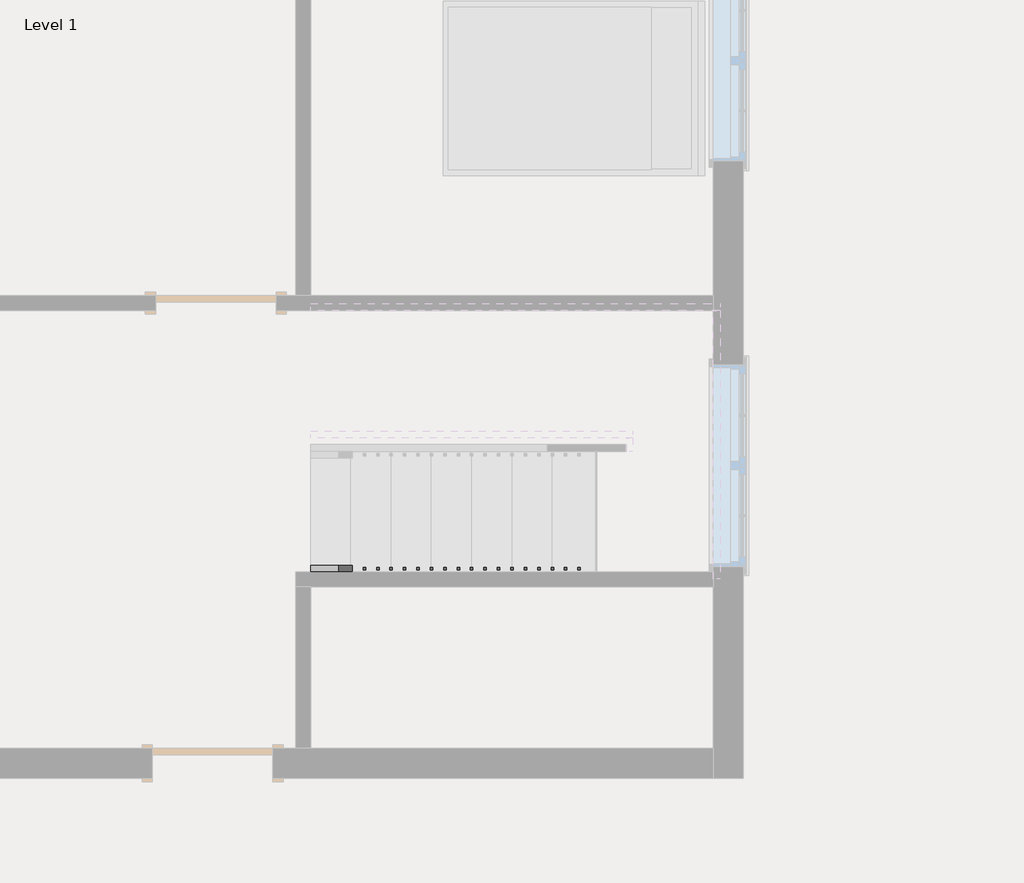
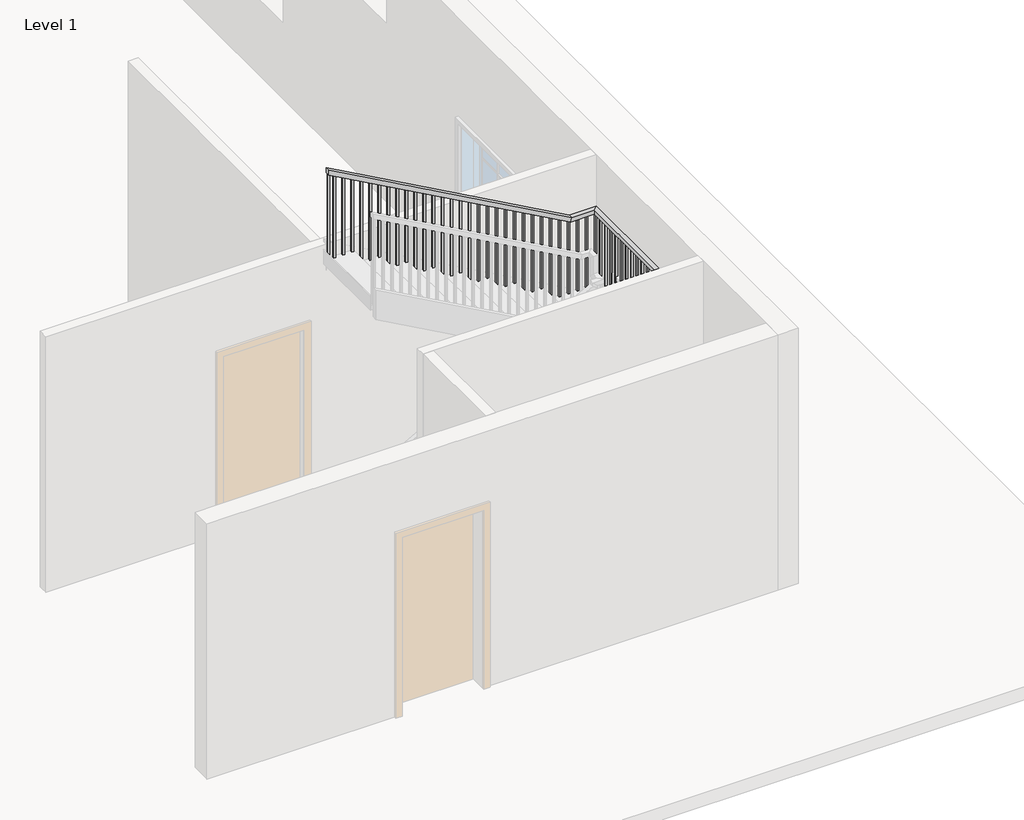
# One storey, part 2 of 3: 1 railing.
"""IFC4 building model written with IfcOpenShell, lengths in millimetres."""

from ifc_helpers import new_model, si_unit, frame, origin, place, context, project, spatial, polyline, outline, extrude, faceted_brep, element, save

model = new_model("IFC4")

# Units and contexts
model_context = context("Model", 3, world=origin())
ifc_project = project(units=[si_unit("LENGTHUNIT", "METRE", prefix="MILLI")], contexts=[model_context])

# Site, building, storey
site = spatial("IfcSite", under=ifc_project)
building = spatial("IfcBuilding", under=site)
storey = spatial("IfcBuildingStorey", under=building, Name="Level 1", Elevation=0.0)

# Railing
placement = place(None, origin())
element("IfcRailing", 1, ObjectType="Handrail - Rectangular", at=placement, inside=storey, context=model_context, shape_type="SolidModel", body=[
    faceted_brep([(-1197.97188, -4765.70869, 1083.7333333), (-1197.97188, -4765.70869, 1025.620221), (-1197.97188, -4816.50869, 1025.620221), (-1197.97188, -4816.50869, 1083.7333333), (1240.42812, -4765.70869, 2438.4), (1253.5917222, -4765.70869, 2387.6), (1253.5917222, -4816.50869, 2387.6), (1240.42812, -4816.50869, 2438.4), (1799.22812, -4765.70869, 2438.4), (1799.22812, -4765.70869, 2387.6), (1850.02812, -4816.50869, 2387.6), (1850.02812, -4816.50869, 2438.4), (1799.22812, -2886.10869, 2438.4), (1799.22812, -2886.10869, 2387.6), (1850.02812, -2835.30869, 2387.6), (1850.02812, -2835.30869, 2438.4), (1545.22812, -2886.10869, 2438.4), (1532.0645177, -2886.10869, 2387.6), (1532.0645177, -2835.30869, 2387.6), (1545.22812, -2835.30869, 2438.4), (-1197.97188, -2886.10869, 3962.4), (-1197.97188, -2835.30869, 3962.4), (-1197.97188, -2835.30869, 3904.2868876), (-1197.97188, -2886.10869, 3904.2868876)], [[[0, 1, 2, 3]], [[1, 0, 4, 5]], [[2, 1, 5, 6]], [[3, 2, 6, 7]], [[0, 3, 7, 4]], [[5, 4, 8, 9]], [[6, 5, 9, 10]], [[7, 6, 10, 11]], [[4, 7, 11, 8]], [[9, 8, 12, 13]], [[10, 9, 13, 14]], [[11, 10, 14, 15]], [[8, 11, 15, 12]], [[13, 12, 16, 17]], [[14, 13, 17, 18]], [[15, 14, 18, 19]], [[12, 15, 19, 16]], [[20, 21, 22, 23]], [[17, 16, 20, 23]], [[18, 17, 23, 22]], [[19, 18, 22, 21]], [[16, 19, 21, 20]]]),
    extrude(outline(polyline([(3856.6618876, -1112.24688), (3867.245221, -1131.29688), (2878.6666667, -1131.29688), (2878.6666667, -1112.24688), (3856.6618876, -1112.24688)])), frame((0.0, -2870.23369, 0.0), z_axis=(0.0, 1.0, 0.0), x_axis=(0.0, 0.0, 1.0)), (0.0, 0.0, 1.0), 19.05),
    extrude(outline(polyline([(3800.2174432, -1010.64688), (3810.8007765, -1029.69688), (2878.6666667, -1029.69688), (2878.6666667, -1010.64688), (3800.2174432, -1010.64688)])), frame((0.0, -2870.23369, 0.0), z_axis=(0.0, 1.0, 0.0), x_axis=(0.0, 0.0, 1.0)), (0.0, 0.0, 1.0), 19.05),
    extrude(outline(polyline([(3743.7729988, -909.04688), (3754.3563321, -928.09688), (2878.6666667, -928.09688), (2878.6666667, -909.04688), (3743.7729988, -909.04688)])), frame((0.0, -2870.23369, 0.0), z_axis=(0.0, 1.0, 0.0), x_axis=(0.0, 0.0, 1.0)), (0.0, 0.0, 1.0), 19.05),
    extrude(outline(polyline([(3687.3285543, -807.44688), (3697.9118876, -826.49688), (2709.3333333, -826.49688), (2709.3333333, -807.44688), (3687.3285543, -807.44688)])), frame((0.0, -2870.23369, 0.0), z_axis=(0.0, 1.0, 0.0), x_axis=(0.0, 0.0, 1.0)), (0.0, 0.0, 1.0), 19.05),
    extrude(outline(polyline([(3630.8841099, -705.84688), (3641.4674432, -724.89688), (2709.3333333, -724.89688), (2709.3333333, -705.84688), (3630.8841099, -705.84688)])), frame((0.0, -2870.23369, 0.0), z_axis=(0.0, 1.0, 0.0), x_axis=(0.0, 0.0, 1.0)), (0.0, 0.0, 1.0), 19.05),
    extrude(outline(polyline([(3574.4396654, -604.24688), (3585.0229988, -623.29688), (2709.3333333, -623.29688), (2709.3333333, -604.24688), (3574.4396654, -604.24688)])), frame((0.0, -2870.23369, 0.0), z_axis=(0.0, 1.0, 0.0), x_axis=(0.0, 0.0, 1.0)), (0.0, 0.0, 1.0), 19.05),
    extrude(outline(polyline([(3517.995221, -502.64688), (3528.5785543, -521.69688), (2540.0, -521.69688), (2540.0, -502.64688), (3517.995221, -502.64688)])), frame((0.0, -2870.23369, 0.0), z_axis=(0.0, 1.0, 0.0), x_axis=(0.0, 0.0, 1.0)), (0.0, 0.0, 1.0), 19.05),
    extrude(outline(polyline([(3461.5507765, -401.04688), (3472.1341099, -420.09688), (2540.0, -420.09688), (2540.0, -401.04688), (3461.5507765, -401.04688)])), frame((0.0, -2870.23369, 0.0), z_axis=(0.0, 1.0, 0.0), x_axis=(0.0, 0.0, 1.0)), (0.0, 0.0, 1.0), 19.05),
    extrude(outline(polyline([(3405.1063321, -299.44688), (3415.6896654, -318.49688), (2540.0, -318.49688), (2540.0, -299.44688), (3405.1063321, -299.44688)])), frame((0.0, -2870.23369, 0.0), z_axis=(0.0, 1.0, 0.0), x_axis=(0.0, 0.0, 1.0)), (0.0, 0.0, 1.0), 19.05),
    extrude(outline(polyline([(3348.6618876, -197.84688), (3359.245221, -216.89688), (2370.6666667, -216.89688), (2370.6666667, -197.84688), (3348.6618876, -197.84688)])), frame((0.0, -2870.23369, 0.0), z_axis=(0.0, 1.0, 0.0), x_axis=(0.0, 0.0, 1.0)), (0.0, 0.0, 1.0), 19.05),
    extrude(outline(polyline([(3292.2174432, -96.24688), (3302.8007765, -115.29688), (2370.6666667, -115.29688), (2370.6666667, -96.24688), (3292.2174432, -96.24688)])), frame((0.0, -2870.23369, 0.0), z_axis=(0.0, 1.0, 0.0), x_axis=(0.0, 0.0, 1.0)), (0.0, 0.0, 1.0), 19.05),
    extrude(outline(polyline([(3235.7729988, 5.35312), (3246.3563321, -13.69688), (2370.6666667, -13.69688), (2370.6666667, 5.35312), (3235.7729988, 5.35312)])), frame((0.0, -2870.23369, 0.0), z_axis=(0.0, 1.0, 0.0), x_axis=(0.0, 0.0, 1.0)), (0.0, 0.0, 1.0), 19.05),
    extrude(outline(polyline([(3179.3285543, 106.95312), (3189.9118876, 87.90312), (2201.3333333, 87.90312), (2201.3333333, 106.95312), (3179.3285543, 106.95312)])), frame((0.0, -2870.23369, 0.0), z_axis=(0.0, 1.0, 0.0), x_axis=(0.0, 0.0, 1.0)), (0.0, 0.0, 1.0), 19.05),
    extrude(outline(polyline([(3122.8841099, 208.55312), (3133.4674432, 189.50312), (2201.3333333, 189.50312), (2201.3333333, 208.55312), (3122.8841099, 208.55312)])), frame((0.0, -2870.23369, 0.0), z_axis=(0.0, 1.0, 0.0), x_axis=(0.0, 0.0, 1.0)), (0.0, 0.0, 1.0), 19.05),
    extrude(outline(polyline([(3066.4396654, 310.15312), (3077.0229988, 291.10312), (2201.3333333, 291.10312), (2201.3333333, 310.15312), (3066.4396654, 310.15312)])), frame((0.0, -2870.23369, 0.0), z_axis=(0.0, 1.0, 0.0), x_axis=(0.0, 0.0, 1.0)), (0.0, 0.0, 1.0), 19.05),
    extrude(outline(polyline([(3009.995221, 411.75312), (3020.5785543, 392.70312), (2032.0, 392.70312), (2032.0, 411.75312), (3009.995221, 411.75312)])), frame((0.0, -2870.23369, 0.0), z_axis=(0.0, 1.0, 0.0), x_axis=(0.0, 0.0, 1.0)), (0.0, 0.0, 1.0), 19.05),
    extrude(outline(polyline([(2953.5507765, 513.35312), (2964.1341099, 494.30312), (2032.0, 494.30312), (2032.0, 513.35312), (2953.5507765, 513.35312)])), frame((0.0, -2870.23369, 0.0), z_axis=(0.0, 1.0, 0.0), x_axis=(0.0, 0.0, 1.0)), (0.0, 0.0, 1.0), 19.05),
    extrude(outline(polyline([(2897.1063321, 614.95312), (2907.6896654, 595.90312), (2032.0, 595.90312), (2032.0, 614.95312), (2897.1063321, 614.95312)])), frame((0.0, -2870.23369, 0.0), z_axis=(0.0, 1.0, 0.0), x_axis=(0.0, 0.0, 1.0)), (0.0, 0.0, 1.0), 19.05),
    extrude(outline(polyline([(2840.6618876, 716.55312), (2851.245221, 697.50312), (1862.6666667, 697.50312), (1862.6666667, 716.55312), (2840.6618876, 716.55312)])), frame((0.0, -2870.23369, 0.0), z_axis=(0.0, 1.0, 0.0), x_axis=(0.0, 0.0, 1.0)), (0.0, 0.0, 1.0), 19.05),
    extrude(outline(polyline([(2784.2174432, 818.15312), (2794.8007765, 799.10312), (1862.6666667, 799.10312), (1862.6666667, 818.15312), (2784.2174432, 818.15312)])), frame((0.0, -2870.23369, 0.0), z_axis=(0.0, 1.0, 0.0), x_axis=(0.0, 0.0, 1.0)), (0.0, 0.0, 1.0), 19.05),
    extrude(outline(polyline([(2727.7729988, 919.75312), (2738.3563321, 900.70312), (1862.6666667, 900.70312), (1862.6666667, 919.75312), (2727.7729988, 919.75312)])), frame((0.0, -2870.23369, 0.0), z_axis=(0.0, 1.0, 0.0), x_axis=(0.0, 0.0, 1.0)), (0.0, 0.0, 1.0), 19.05),
    extrude(outline(polyline([(2671.3285543, 1021.35312), (2681.9118876, 1002.30312), (1693.3333333, 1002.30312), (1693.3333333, 1021.35312), (2671.3285543, 1021.35312)])), frame((0.0, -2870.23369, 0.0), z_axis=(0.0, 1.0, 0.0), x_axis=(0.0, 0.0, 1.0)), (0.0, 0.0, 1.0), 19.05),
    extrude(outline(polyline([(2614.8841099, 1122.95312), (2625.4674432, 1103.90312), (1693.3333333, 1103.90312), (1693.3333333, 1122.95312), (2614.8841099, 1122.95312)])), frame((0.0, -2870.23369, 0.0), z_axis=(0.0, 1.0, 0.0), x_axis=(0.0, 0.0, 1.0)), (0.0, 0.0, 1.0), 19.05),
    extrude(outline(polyline([(2558.4396654, 1224.55312), (2569.0229988, 1205.50312), (1693.3333333, 1205.50312), (1693.3333333, 1224.55312), (2558.4396654, 1224.55312)])), frame((0.0, -2870.23369, 0.0), z_axis=(0.0, 1.0, 0.0), x_axis=(0.0, 0.0, 1.0)), (0.0, 0.0, 1.0), 19.05),
    extrude(outline(polyline([(2501.995221, 1326.15312), (2512.5785543, 1307.10312), (1524.0, 1307.10312), (1524.0, 1326.15312), (2501.995221, 1326.15312)])), frame((0.0, -2870.23369, 0.0), z_axis=(0.0, 1.0, 0.0), x_axis=(0.0, 0.0, 1.0)), (0.0, 0.0, 1.0), 19.05),
    extrude(outline(polyline([(2445.5507765, 1427.75312), (2456.1341099, 1408.70312), (1524.0, 1408.70312), (1524.0, 1427.75312), (2445.5507765, 1427.75312)])), frame((0.0, -2870.23369, 0.0), z_axis=(0.0, 1.0, 0.0), x_axis=(0.0, 0.0, 1.0)), (0.0, 0.0, 1.0), 19.05),
    extrude(outline(polyline([(2389.1063321, 1529.35312), (2399.6896654, 1510.30312), (1524.0, 1510.30312), (1524.0, 1529.35312), (2389.1063321, 1529.35312)])), frame((0.0, -2870.23369, 0.0), z_axis=(0.0, 1.0, 0.0), x_axis=(0.0, 0.0, 1.0)), (0.0, 0.0, 1.0), 19.05),
    extrude(outline(polyline([(1630.95312, -2851.18369), (1630.95312, -2870.23369), (1611.90312, -2870.23369), (1611.90312, -2851.18369), (1630.95312, -2851.18369)])), frame((0.0, 0.0, 1524.0), z_axis=(0.0, 0.0, 1.0), x_axis=(1.0, 0.0, 0.0)), (0.0, 0.0, 1.0), 863.6),
    extrude(outline(polyline([(1732.55312, -2851.18369), (1732.55312, -2870.23369), (1713.50312, -2870.23369), (1713.50312, -2851.18369), (1732.55312, -2851.18369)])), frame((0.0, 0.0, 1524.0), z_axis=(0.0, 0.0, 1.0), x_axis=(1.0, 0.0, 0.0)), (0.0, 0.0, 1.0), 863.6),
    extrude(outline(polyline([(1834.15312, -2971.83369), (1815.10312, -2971.83369), (1815.10312, -2952.78369), (1834.15312, -2952.78369), (1834.15312, -2971.83369)])), frame((0.0, 0.0, 1524.0), z_axis=(0.0, 0.0, 1.0), x_axis=(1.0, 0.0, 0.0)), (0.0, 0.0, 1.0), 863.6),
    extrude(outline(polyline([(1834.15312, -3073.43369), (1815.10312, -3073.43369), (1815.10312, -3054.38369), (1834.15312, -3054.38369), (1834.15312, -3073.43369)])), frame((0.0, 0.0, 1524.0), z_axis=(0.0, 0.0, 1.0), x_axis=(1.0, 0.0, 0.0)), (0.0, 0.0, 1.0), 863.6),
    extrude(outline(polyline([(1834.15312, -3175.03369), (1815.10312, -3175.03369), (1815.10312, -3155.98369), (1834.15312, -3155.98369), (1834.15312, -3175.03369)])), frame((0.0, 0.0, 1524.0), z_axis=(0.0, 0.0, 1.0), x_axis=(1.0, 0.0, 0.0)), (0.0, 0.0, 1.0), 863.6),
    extrude(outline(polyline([(1834.15312, -3276.63369), (1815.10312, -3276.63369), (1815.10312, -3257.58369), (1834.15312, -3257.58369), (1834.15312, -3276.63369)])), frame((0.0, 0.0, 1524.0), z_axis=(0.0, 0.0, 1.0), x_axis=(1.0, 0.0, 0.0)), (0.0, 0.0, 1.0), 863.6),
    extrude(outline(polyline([(1834.15312, -3378.23369), (1815.10312, -3378.23369), (1815.10312, -3359.18369), (1834.15312, -3359.18369), (1834.15312, -3378.23369)])), frame((0.0, 0.0, 1524.0), z_axis=(0.0, 0.0, 1.0), x_axis=(1.0, 0.0, 0.0)), (0.0, 0.0, 1.0), 863.6),
    extrude(outline(polyline([(1834.15312, -3479.83369), (1815.10312, -3479.83369), (1815.10312, -3460.78369), (1834.15312, -3460.78369), (1834.15312, -3479.83369)])), frame((0.0, 0.0, 1524.0), z_axis=(0.0, 0.0, 1.0), x_axis=(1.0, 0.0, 0.0)), (0.0, 0.0, 1.0), 863.6),
    extrude(outline(polyline([(1834.15312, -3581.43369), (1815.10312, -3581.43369), (1815.10312, -3562.38369), (1834.15312, -3562.38369), (1834.15312, -3581.43369)])), frame((0.0, 0.0, 1524.0), z_axis=(0.0, 0.0, 1.0), x_axis=(1.0, 0.0, 0.0)), (0.0, 0.0, 1.0), 863.6),
    extrude(outline(polyline([(1834.15312, -3683.03369), (1815.10312, -3683.03369), (1815.10312, -3663.98369), (1834.15312, -3663.98369), (1834.15312, -3683.03369)])), frame((0.0, 0.0, 1524.0), z_axis=(0.0, 0.0, 1.0), x_axis=(1.0, 0.0, 0.0)), (0.0, 0.0, 1.0), 863.6),
    extrude(outline(polyline([(1834.15312, -3784.63369), (1815.10312, -3784.63369), (1815.10312, -3765.58369), (1834.15312, -3765.58369), (1834.15312, -3784.63369)])), frame((0.0, 0.0, 1524.0), z_axis=(0.0, 0.0, 1.0), x_axis=(1.0, 0.0, 0.0)), (0.0, 0.0, 1.0), 863.6),
    extrude(outline(polyline([(1834.15312, -3886.23369), (1815.10312, -3886.23369), (1815.10312, -3867.18369), (1834.15312, -3867.18369), (1834.15312, -3886.23369)])), frame((0.0, 0.0, 1524.0), z_axis=(0.0, 0.0, 1.0), x_axis=(1.0, 0.0, 0.0)), (0.0, 0.0, 1.0), 863.6),
    extrude(outline(polyline([(1834.15312, -3987.83369), (1815.10312, -3987.83369), (1815.10312, -3968.78369), (1834.15312, -3968.78369), (1834.15312, -3987.83369)])), frame((0.0, 0.0, 1524.0), z_axis=(0.0, 0.0, 1.0), x_axis=(1.0, 0.0, 0.0)), (0.0, 0.0, 1.0), 863.6),
    extrude(outline(polyline([(1834.15312, -4089.43369), (1815.10312, -4089.43369), (1815.10312, -4070.38369), (1834.15312, -4070.38369), (1834.15312, -4089.43369)])), frame((0.0, 0.0, 1524.0), z_axis=(0.0, 0.0, 1.0), x_axis=(1.0, 0.0, 0.0)), (0.0, 0.0, 1.0), 863.6),
    extrude(outline(polyline([(1834.15312, -4191.03369), (1815.10312, -4191.03369), (1815.10312, -4171.98369), (1834.15312, -4171.98369), (1834.15312, -4191.03369)])), frame((0.0, 0.0, 1524.0), z_axis=(0.0, 0.0, 1.0), x_axis=(1.0, 0.0, 0.0)), (0.0, 0.0, 1.0), 863.6),
    extrude(outline(polyline([(1834.15312, -4292.63369), (1815.10312, -4292.63369), (1815.10312, -4273.58369), (1834.15312, -4273.58369), (1834.15312, -4292.63369)])), frame((0.0, 0.0, 1524.0), z_axis=(0.0, 0.0, 1.0), x_axis=(1.0, 0.0, 0.0)), (0.0, 0.0, 1.0), 863.6),
    extrude(outline(polyline([(1834.15312, -4394.23369), (1815.10312, -4394.23369), (1815.10312, -4375.18369), (1834.15312, -4375.18369), (1834.15312, -4394.23369)])), frame((0.0, 0.0, 1524.0), z_axis=(0.0, 0.0, 1.0), x_axis=(1.0, 0.0, 0.0)), (0.0, 0.0, 1.0), 863.6),
    extrude(outline(polyline([(1834.15312, -4495.83369), (1815.10312, -4495.83369), (1815.10312, -4476.78369), (1834.15312, -4476.78369), (1834.15312, -4495.83369)])), frame((0.0, 0.0, 1524.0), z_axis=(0.0, 0.0, 1.0), x_axis=(1.0, 0.0, 0.0)), (0.0, 0.0, 1.0), 863.6),
    extrude(outline(polyline([(1834.15312, -4597.43369), (1815.10312, -4597.43369), (1815.10312, -4578.38369), (1834.15312, -4578.38369), (1834.15312, -4597.43369)])), frame((0.0, 0.0, 1524.0), z_axis=(0.0, 0.0, 1.0), x_axis=(1.0, 0.0, 0.0)), (0.0, 0.0, 1.0), 863.6),
    extrude(outline(polyline([(1834.15312, -4699.03369), (1815.10312, -4699.03369), (1815.10312, -4679.98369), (1834.15312, -4679.98369), (1834.15312, -4699.03369)])), frame((0.0, 0.0, 1524.0), z_axis=(0.0, 0.0, 1.0), x_axis=(1.0, 0.0, 0.0)), (0.0, 0.0, 1.0), 863.6),
    extrude(outline(polyline([(1738.90312, -4800.63369), (1738.90312, -4781.58369), (1757.95312, -4781.58369), (1757.95312, -4800.63369), (1738.90312, -4800.63369)])), frame((0.0, 0.0, 1524.0), z_axis=(0.0, 0.0, 1.0), x_axis=(1.0, 0.0, 0.0)), (0.0, 0.0, 1.0), 863.6),
    extrude(outline(polyline([(1637.30312, -4800.63369), (1637.30312, -4781.58369), (1656.35312, -4781.58369), (1656.35312, -4800.63369), (1637.30312, -4800.63369)])), frame((0.0, 0.0, 1524.0), z_axis=(0.0, 0.0, 1.0), x_axis=(1.0, 0.0, 0.0)), (0.0, 0.0, 1.0), 863.6),
    extrude(outline(polyline([(1535.70312, -4800.63369), (1535.70312, -4781.58369), (1554.75312, -4781.58369), (1554.75312, -4800.63369), (1535.70312, -4800.63369)])), frame((0.0, 0.0, 1524.0), z_axis=(0.0, 0.0, 1.0), x_axis=(1.0, 0.0, 0.0)), (0.0, 0.0, 1.0), 863.6),
    extrude(outline(polyline([(1434.10312, -4800.63369), (1434.10312, -4781.58369), (1453.15312, -4781.58369), (1453.15312, -4800.63369), (1434.10312, -4800.63369)])), frame((0.0, 0.0, 1524.0), z_axis=(0.0, 0.0, 1.0), x_axis=(1.0, 0.0, 0.0)), (0.0, 0.0, 1.0), 863.6),
    extrude(outline(polyline([(1332.50312, -4800.63369), (1332.50312, -4781.58369), (1351.55312, -4781.58369), (1351.55312, -4800.63369), (1332.50312, -4800.63369)])), frame((0.0, 0.0, 1524.0), z_axis=(0.0, 0.0, 1.0), x_axis=(1.0, 0.0, 0.0)), (0.0, 0.0, 1.0), 863.6),
    extrude(outline(polyline([(2385.5785543, 1249.95312), (2374.995221, 1230.90312), (1524.0, 1230.90312), (1524.0, 1249.95312), (2385.5785543, 1249.95312)])), frame((0.0, -4800.63369, 0.0), z_axis=(0.0, 1.0, 0.0), x_axis=(0.0, 0.0, 1.0)), (0.0, 0.0, 1.0), 19.05),
    extrude(outline(polyline([(2329.1341099, 1148.35312), (2318.5507765, 1129.30312), (1354.6666667, 1129.30312), (1354.6666667, 1148.35312), (2329.1341099, 1148.35312)])), frame((0.0, -4800.63369, 0.0), z_axis=(0.0, 1.0, 0.0), x_axis=(0.0, 0.0, 1.0)), (0.0, 0.0, 1.0), 19.05),
    extrude(outline(polyline([(2272.6896654, 1046.75312), (2262.1063321, 1027.70312), (1354.6666667, 1027.70312), (1354.6666667, 1046.75312), (2272.6896654, 1046.75312)])), frame((0.0, -4800.63369, 0.0), z_axis=(0.0, 1.0, 0.0), x_axis=(0.0, 0.0, 1.0)), (0.0, 0.0, 1.0), 19.05),
    extrude(outline(polyline([(2216.245221, 945.15312), (2205.6618876, 926.10312), (1354.6666667, 926.10312), (1354.6666667, 945.15312), (2216.245221, 945.15312)])), frame((0.0, -4800.63369, 0.0), z_axis=(0.0, 1.0, 0.0), x_axis=(0.0, 0.0, 1.0)), (0.0, 0.0, 1.0), 19.05),
    extrude(outline(polyline([(2159.8007765, 843.55312), (2149.2174432, 824.50312), (1185.3333333, 824.50312), (1185.3333333, 843.55312), (2159.8007765, 843.55312)])), frame((0.0, -4800.63369, 0.0), z_axis=(0.0, 1.0, 0.0), x_axis=(0.0, 0.0, 1.0)), (0.0, 0.0, 1.0), 19.05),
    extrude(outline(polyline([(2103.3563321, 741.95312), (2092.7729988, 722.90312), (1185.3333333, 722.90312), (1185.3333333, 741.95312), (2103.3563321, 741.95312)])), frame((0.0, -4800.63369, 0.0), z_axis=(0.0, 1.0, 0.0), x_axis=(0.0, 0.0, 1.0)), (0.0, 0.0, 1.0), 19.05),
    extrude(outline(polyline([(2046.9118876, 640.35312), (2036.3285543, 621.30312), (1185.3333333, 621.30312), (1185.3333333, 640.35312), (2046.9118876, 640.35312)])), frame((0.0, -4800.63369, 0.0), z_axis=(0.0, 1.0, 0.0), x_axis=(0.0, 0.0, 1.0)), (0.0, 0.0, 1.0), 19.05),
    extrude(outline(polyline([(1990.4674432, 538.75312), (1979.8841099, 519.70312), (1016.0, 519.70312), (1016.0, 538.75312), (1990.4674432, 538.75312)])), frame((0.0, -4800.63369, 0.0), z_axis=(0.0, 1.0, 0.0), x_axis=(0.0, 0.0, 1.0)), (0.0, 0.0, 1.0), 19.05),
    extrude(outline(polyline([(1934.0229988, 437.15312), (1923.4396654, 418.10312), (1016.0, 418.10312), (1016.0, 437.15312), (1934.0229988, 437.15312)])), frame((0.0, -4800.63369, 0.0), z_axis=(0.0, 1.0, 0.0), x_axis=(0.0, 0.0, 1.0)), (0.0, 0.0, 1.0), 19.05),
    extrude(outline(polyline([(1877.5785543, 335.55312), (1866.995221, 316.50312), (1016.0, 316.50312), (1016.0, 335.55312), (1877.5785543, 335.55312)])), frame((0.0, -4800.63369, 0.0), z_axis=(0.0, 1.0, 0.0), x_axis=(0.0, 0.0, 1.0)), (0.0, 0.0, 1.0), 19.05),
    extrude(outline(polyline([(1821.1341099, 233.95312), (1810.5507765, 214.90312), (846.6666667, 214.90312), (846.6666667, 233.95312), (1821.1341099, 233.95312)])), frame((0.0, -4800.63369, 0.0), z_axis=(0.0, 1.0, 0.0), x_axis=(0.0, 0.0, 1.0)), (0.0, 0.0, 1.0), 19.05),
    extrude(outline(polyline([(1764.6896654, 132.35312), (1754.1063321, 113.30312), (846.6666667, 113.30312), (846.6666667, 132.35312), (1764.6896654, 132.35312)])), frame((0.0, -4800.63369, 0.0), z_axis=(0.0, 1.0, 0.0), x_axis=(0.0, 0.0, 1.0)), (0.0, 0.0, 1.0), 19.05),
    extrude(outline(polyline([(1708.245221, 30.75312), (1697.6618876, 11.70312), (846.6666667, 11.70312), (846.6666667, 30.75312), (1708.245221, 30.75312)])), frame((0.0, -4800.63369, 0.0), z_axis=(0.0, 1.0, 0.0), x_axis=(0.0, 0.0, 1.0)), (0.0, 0.0, 1.0), 19.05),
    extrude(outline(polyline([(1651.8007765, -70.84688), (1641.2174432, -89.89688), (677.3333333, -89.89688), (677.3333333, -70.84688), (1651.8007765, -70.84688)])), frame((0.0, -4800.63369, 0.0), z_axis=(0.0, 1.0, 0.0), x_axis=(0.0, 0.0, 1.0)), (0.0, 0.0, 1.0), 19.05),
    extrude(outline(polyline([(1595.3563321, -172.44688), (1584.7729988, -191.49688), (677.3333333, -191.49688), (677.3333333, -172.44688), (1595.3563321, -172.44688)])), frame((0.0, -4800.63369, 0.0), z_axis=(0.0, 1.0, 0.0), x_axis=(0.0, 0.0, 1.0)), (0.0, 0.0, 1.0), 19.05),
    extrude(outline(polyline([(1538.9118876, -274.04688), (1528.3285543, -293.09688), (677.3333333, -293.09688), (677.3333333, -274.04688), (1538.9118876, -274.04688)])), frame((0.0, -4800.63369, 0.0), z_axis=(0.0, 1.0, 0.0), x_axis=(0.0, 0.0, 1.0)), (0.0, 0.0, 1.0), 19.05),
    extrude(outline(polyline([(1482.4674432, -375.64688), (1471.8841099, -394.69688), (508.0, -394.69688), (508.0, -375.64688), (1482.4674432, -375.64688)])), frame((0.0, -4800.63369, 0.0), z_axis=(0.0, 1.0, 0.0), x_axis=(0.0, 0.0, 1.0)), (0.0, 0.0, 1.0), 19.05),
    extrude(outline(polyline([(1426.0229988, -477.24688), (1415.4396654, -496.29688), (508.0, -496.29688), (508.0, -477.24688), (1426.0229988, -477.24688)])), frame((0.0, -4800.63369, 0.0), z_axis=(0.0, 1.0, 0.0), x_axis=(0.0, 0.0, 1.0)), (0.0, 0.0, 1.0), 19.05),
    extrude(outline(polyline([(1369.5785543, -578.84688), (1358.995221, -597.89688), (508.0, -597.89688), (508.0, -578.84688), (1369.5785543, -578.84688)])), frame((0.0, -4800.63369, 0.0), z_axis=(0.0, 1.0, 0.0), x_axis=(0.0, 0.0, 1.0)), (0.0, 0.0, 1.0), 19.05),
    extrude(outline(polyline([(1313.1341099, -680.44688), (1302.5507765, -699.49688), (338.6666667, -699.49688), (338.6666667, -680.44688), (1313.1341099, -680.44688)])), frame((0.0, -4800.63369, 0.0), z_axis=(0.0, 1.0, 0.0), x_axis=(0.0, 0.0, 1.0)), (0.0, 0.0, 1.0), 19.05),
    extrude(outline(polyline([(1256.6896654, -782.04688), (1246.1063321, -801.09688), (338.6666667, -801.09688), (338.6666667, -782.04688), (1256.6896654, -782.04688)])), frame((0.0, -4800.63369, 0.0), z_axis=(0.0, 1.0, 0.0), x_axis=(0.0, 0.0, 1.0)), (0.0, 0.0, 1.0), 19.05),
    extrude(outline(polyline([(1200.245221, -883.64688), (1189.6618876, -902.69688), (338.6666667, -902.69688), (338.6666667, -883.64688), (1200.245221, -883.64688)])), frame((0.0, -4800.63369, 0.0), z_axis=(0.0, 1.0, 0.0), x_axis=(0.0, 0.0, 1.0)), (0.0, 0.0, 1.0), 19.05),
    extrude(outline(polyline([(1143.8007765, -985.24688), (1133.2174432, -1004.29688), (169.3333333, -1004.29688), (169.3333333, -985.24688), (1143.8007765, -985.24688)])), frame((0.0, -4800.63369, 0.0), z_axis=(0.0, 1.0, 0.0), x_axis=(0.0, 0.0, 1.0)), (0.0, 0.0, 1.0), 19.05),
    extrude(outline(polyline([(1087.3563321, -1086.84688), (1076.7729988, -1105.89688), (169.3333333, -1105.89688), (169.3333333, -1086.84688), (1087.3563321, -1086.84688)])), frame((0.0, -4800.63369, 0.0), z_axis=(0.0, 1.0, 0.0), x_axis=(0.0, 0.0, 1.0)), (0.0, 0.0, 1.0), 19.05),
    extrude(outline(polyline([(1834.15312, -2870.23369), (1815.10312, -2870.23369), (1815.10312, -2851.18369), (1834.15312, -2851.18369), (1834.15312, -2870.23369)])), frame((0.0, 0.0, 1524.0), z_axis=(0.0, 0.0, 1.0), x_axis=(1.0, 0.0, 0.0)), (0.0, 0.0, 1.0), 863.6),
    extrude(outline(polyline([(1815.10312, -4800.63369), (1815.10312, -4781.58369), (1834.15312, -4781.58369), (1834.15312, -4800.63369), (1815.10312, -4800.63369)])), frame((0.0, 0.0, 1524.0), z_axis=(0.0, 0.0, 1.0), x_axis=(1.0, 0.0, 0.0)), (0.0, 0.0, 1.0), 863.6),
    extrude(outline(polyline([(3893.7035543, -1178.92188), (3904.2868876, -1197.97188), (2878.6666667, -1197.97188), (2878.6666667, -1178.92188), (3893.7035543, -1178.92188)])), frame((0.0, -2870.23369, 0.0), z_axis=(0.0, 1.0, 0.0), x_axis=(0.0, 0.0, 1.0)), (0.0, 0.0, 1.0), 19.05),
    extrude(outline(polyline([(1036.2035543, -1178.92188), (1025.620221, -1197.97188), (169.3333333, -1197.97188), (169.3333333, -1178.92188), (1036.2035543, -1178.92188)])), frame((0.0, -4800.63369, 0.0), z_axis=(0.0, 1.0, 0.0), x_axis=(0.0, 0.0, 1.0)), (0.0, 0.0, 1.0), 19.05),
])

save(model, "model.ifc")

# Revit data of these elements
# Type "Handrail - Rectangular"
#   Assembly Code = "C2010400"
#   built-in parameter 1008612 = 0.0416667 (stored number, unit not read)
#   built-in parameter 1008611 = 0.0416667 (stored number, unit not read)
#   built-in parameter 1008609 = 0.333333 (stored number, unit not read)
#   built-in parameter 1008604 = 0.166667 (stored number, unit not read)
#   built-in parameter 1008603 = 0.166667 (stored number, unit not read)
#   Railing Height = 3' - 0"
#   built-in parameter 1008630 = 2
#   built-in parameter 1008610 = 2
#   built-in parameter 1008618 = Baluster - Square : 3/4"
# Element 1 (IfcRailing, "Handrail - Rectangular")
#   Phase Created = New Construction
